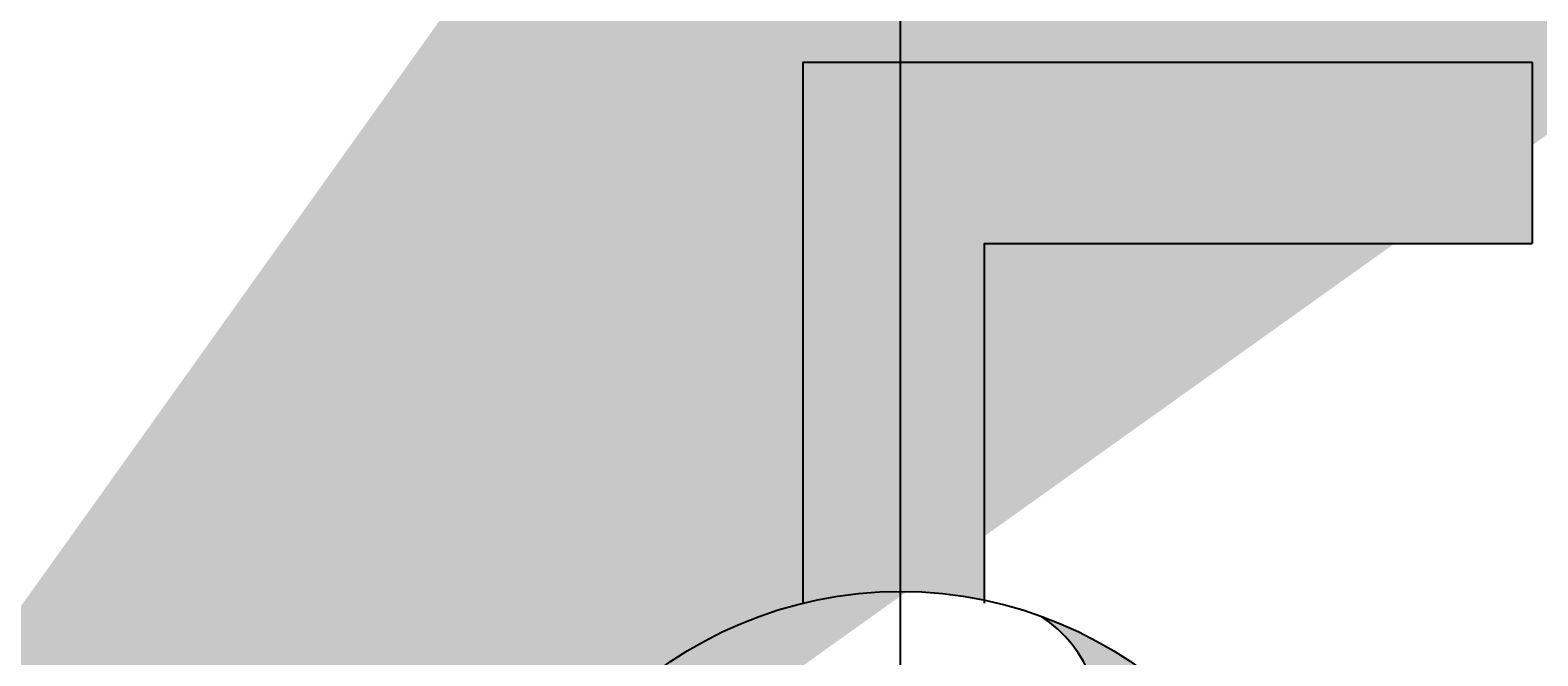
# Model space of a CAD drawing. Units: millimetres. Extents: x -22994 to 29398, y -19990 to 20176.
# Tile 118 of 135: x 204 to 245, y 156 to 174. Entities that reach past the tile are written whole.
import ezdxf

# ---------------------------------------------------------------- set-up
doc = ezdxf.new("R2010")
doc.units = ezdxf.units.MM
doc.header["$MEASUREMENT"] = 0
for name, color, linetype, lineweight in [('M-DIMS', 2, 'Continuous', 18), ('M-EQPM', 7, 'Continuous', 25), ('M-EQPM-PATT', 7, 'Continuous', 18)]:
    doc.layers.add(name, color=color, linetype=linetype, lineweight=lineweight)
doc.styles.get("Standard").update_dxf_attribs({"font": 'arial.ttf'})
doc.dimstyles.get("Standard").update_dxf_attribs({"dimtxt": 0.18, "dimasz": 10000, "dimexe": 0.18, "dimexo": 0.0625, "dimgap": 0.09, "dimtad": 0, "dimtih": 1, "dimtoh": 1, "dimdec": 0, "dimzin": 0, "dimdsep": 46, "dimtxsty": 'Standard', "dimcen": 0.09, "dimadec": 0, "dimazin": 0, "dimtfac": 1, "dimtdec": 0, "dimtofl": 0, "dimtmove": 0, "dimatfit": 3, "dimfxl": 1, "dimtolj": 1, "dimtzin": 0, "dimlwd": 30, "dimarcsym": 0})

# ---------------------------------------------------------------- blocks, each defined once
blk = doc.blocks.new('*D2')
at = {"layer": 'Defpoints', "color": 0, "transparency": 16777216}
for p in [(6.677, 10.271), (290.852, 10.271), (290.852, -5.079)]:
    blk.add_point(p, dxfattribs=at)
at = {"layer": 'M-DIMS', "color": 0, "lineweight": -2, "transparency": 16777216}
for p, q in [((6.677, 10.209), (6.677, -5.259)), ((290.852, 10.209), (290.852, -5.259))]:
    blk.add_line(p, q, dxfattribs=at)
at = {"layer": 'M-DIMS', "color": 0, "lineweight": 30, "transparency": 16777216}
for p, q in [((-9993.323, -5.079), (-19993.323, -5.079)), ((10290.852, -5.079), (20290.852, -5.079))]:
    blk.add_line(p, q, dxfattribs=at)
at = {"layer": 'M-DIMS', "color": 0, "transparency": 16777216}
for points in [[(-9993.323, 1661.588), (-9993.323, -1671.745), (6.677, -5.079)], [(10290.852, 1661.588), (10290.852, -1671.745), (290.852, -5.079)]]:
    blk.add_solid(points, dxfattribs=at)
at = {"layer": 'M-DIMS', "color": 0, "transparency": 16777216, "insert": (148.765, -5.079), "char_height": 0.18, "attachment_point": 5}
blk.add_mtext('\\A1;284.2', dxfattribs=at)
blk = doc.blocks.new('*D3')
at = {"layer": 'Defpoints', "color": 0, "transparency": 16777216}
for p in [(110.265, 204.165), (110.265, 176.366), (95.833, 127.967)]:
    blk.add_point(p, dxfattribs=at)
at = {"layer": 'M-DIMS', "color": 0, "lineweight": 30, "transparency": 16777216}
for p, q in [((-9904.167, 204.165), (-19904.167, 204.165)), ((10110.265, 204.165), (20110.265, 204.165))]:
    blk.add_line(p, q, dxfattribs=at)
at = {"layer": 'M-DIMS', "color": 0, "lineweight": -2, "transparency": 16777216}
for p, q in [((95.833, 128.03), (95.833, 204.345)), ((110.265, 176.429), (110.265, 204.345))]:
    blk.add_line(p, q, dxfattribs=at)
at = {"layer": 'M-DIMS', "color": 0, "transparency": 16777216}
for points in [[(-9904.167, 1870.832), (-9904.167, -1462.501), (95.833, 204.165)], [(10110.265, 1870.832), (10110.265, -1462.501), (110.265, 204.165)]]:
    blk.add_solid(points, dxfattribs=at)
at = {"layer": 'M-DIMS', "color": 0, "transparency": 16777216, "insert": (103.049, 204.165), "char_height": 0.18, "attachment_point": 5}
blk.add_mtext('\\A1;14.432', dxfattribs=at)
blk = doc.blocks.new('*D4')
at = {"layer": 'Defpoints', "color": 0, "transparency": 16777216}
for p in [(116.265, 204.165), (110.265, 176.366), (116.265, 176.366)]:
    blk.add_point(p, dxfattribs=at)
at = {"layer": 'M-DIMS', "color": 0, "lineweight": 30, "transparency": 16777216}
for p, q in [((-9889.735, 204.165), (-19889.735, 204.165)), ((10116.265, 204.165), (20116.265, 204.165))]:
    blk.add_line(p, q, dxfattribs=at)
at = {"layer": 'M-DIMS', "color": 0, "lineweight": -2, "transparency": 16777216}
for p, q in [((110.265, 176.429), (110.265, 204.345)), ((116.265, 176.429), (116.265, 204.345))]:
    blk.add_line(p, q, dxfattribs=at)
at = {"layer": 'M-DIMS', "color": 0, "transparency": 16777216}
for points in [[(-9889.735, 1870.832), (-9889.735, -1462.501), (110.265, 204.165)], [(10116.265, 1870.832), (10116.265, -1462.501), (116.265, 204.165)]]:
    blk.add_solid(points, dxfattribs=at)
at = {"layer": 'M-DIMS', "color": 0, "transparency": 16777216, "insert": (113.265, 204.165), "char_height": 0.18, "attachment_point": 5}
blk.add_mtext('\\A1;6', dxfattribs=at)
blk = doc.blocks.new('*D5')
at = {"layer": 'Defpoints', "color": 0, "transparency": 16777216}
for p in [(181.265, 204.165), (116.265, 176.366), (181.265, 176.366)]:
    blk.add_point(p, dxfattribs=at)
at = {"layer": 'M-DIMS', "color": 0, "lineweight": 30, "transparency": 16777216}
for p, q in [((-9883.735, 204.165), (-19883.735, 204.165)), ((10181.265, 204.165), (20181.265, 204.165))]:
    blk.add_line(p, q, dxfattribs=at)
at = {"layer": 'M-DIMS', "color": 0, "lineweight": -2, "transparency": 16777216}
for p, q in [((116.265, 176.429), (116.265, 204.345)), ((181.265, 176.429), (181.265, 204.345))]:
    blk.add_line(p, q, dxfattribs=at)
at = {"layer": 'M-DIMS', "color": 0, "transparency": 16777216}
for points in [[(-9883.735, 1870.832), (-9883.735, -1462.501), (116.265, 204.165)], [(10181.265, 1870.832), (10181.265, -1462.501), (181.265, 204.165)]]:
    blk.add_solid(points, dxfattribs=at)
at = {"layer": 'M-DIMS', "color": 0, "transparency": 16777216, "insert": (148.765, 204.165), "char_height": 0.18, "attachment_point": 5}
blk.add_mtext('\\A1;65', dxfattribs=at)
blk = doc.blocks.new('*D6')
at = {"layer": 'Defpoints', "color": 0, "transparency": 16777216}
for p in [(187.265, 204.165), (181.265, 176.366), (187.265, 176.366)]:
    blk.add_point(p, dxfattribs=at)
at = {"layer": 'M-DIMS', "color": 0, "lineweight": 30, "transparency": 16777216}
for p, q in [((-9818.735, 204.165), (-19818.735, 204.165)), ((10187.265, 204.165), (20187.265, 204.165))]:
    blk.add_line(p, q, dxfattribs=at)
at = {"layer": 'M-DIMS', "color": 0, "lineweight": -2, "transparency": 16777216}
for p, q in [((181.265, 176.429), (181.265, 204.345)), ((187.265, 176.429), (187.265, 204.345))]:
    blk.add_line(p, q, dxfattribs=at)
at = {"layer": 'M-DIMS', "color": 0, "transparency": 16777216}
for points in [[(-9818.735, 1870.832), (-9818.735, -1462.501), (181.265, 204.165)], [(10187.265, 1870.832), (10187.265, -1462.501), (187.265, 204.165)]]:
    blk.add_solid(points, dxfattribs=at)
at = {"layer": 'M-DIMS', "color": 0, "transparency": 16777216, "insert": (184.265, 204.165), "char_height": 0.18, "attachment_point": 5}
blk.add_mtext('\\A1;6', dxfattribs=at)
blk = doc.blocks.new('*D7')
at = {"layer": 'Defpoints', "color": 0, "transparency": 16777216}
for p in [(201.697, 204.165), (187.265, 176.366), (201.697, 127.967)]:
    blk.add_point(p, dxfattribs=at)
at = {"layer": 'M-DIMS', "color": 0, "lineweight": 30, "transparency": 16777216}
for p, q in [((-9812.735, 204.165), (-19812.735, 204.165)), ((10201.697, 204.165), (20201.697, 204.165))]:
    blk.add_line(p, q, dxfattribs=at)
at = {"layer": 'M-DIMS', "color": 0, "lineweight": -2, "transparency": 16777216}
for p, q in [((187.265, 176.429), (187.265, 204.345)), ((201.697, 128.03), (201.697, 204.345))]:
    blk.add_line(p, q, dxfattribs=at)
at = {"layer": 'M-DIMS', "color": 0, "transparency": 16777216}
for points in [[(-9812.735, 1870.832), (-9812.735, -1462.501), (187.265, 204.165)], [(10201.697, 1870.832), (10201.697, -1462.501), (201.697, 204.165)]]:
    blk.add_solid(points, dxfattribs=at)
at = {"layer": 'M-DIMS', "color": 0, "transparency": 16777216, "insert": (194.481, 204.165), "char_height": 0.18, "attachment_point": 5}
blk.add_mtext('\\A1;14.432', dxfattribs=at)
blk = doc.blocks.new('*D8')
at = {"layer": 'Defpoints', "color": 0, "transparency": 16777216}
for p in [(227.648, 204.165), (227.648, 146.73), (201.697, 127.967)]:
    blk.add_point(p, dxfattribs=at)
at = {"layer": 'M-DIMS', "color": 0, "lineweight": 30, "transparency": 16777216}
for p, q in [((-9798.303, 204.165), (-19798.303, 204.165)), ((10227.648, 204.165), (20227.648, 204.165))]:
    blk.add_line(p, q, dxfattribs=at)
at = {"layer": 'M-DIMS', "color": 0, "lineweight": -2, "transparency": 16777216}
for p, q in [((201.697, 128.03), (201.697, 204.345)), ((227.648, 146.792), (227.648, 204.345))]:
    blk.add_line(p, q, dxfattribs=at)
at = {"layer": 'M-DIMS', "color": 0, "transparency": 16777216}
for points in [[(-9798.303, 1870.832), (-9798.303, -1462.501), (201.697, 204.165)], [(10227.648, 1870.832), (10227.648, -1462.501), (227.648, 204.165)]]:
    blk.add_solid(points, dxfattribs=at)
at = {"layer": 'M-DIMS', "color": 0, "transparency": 16777216, "insert": (214.673, 204.165), "char_height": 0.18, "attachment_point": 5}
blk.add_mtext('\\A1;25.95', dxfattribs=at)
blk = doc.blocks.new('*D9')
at = {"layer": 'Defpoints', "color": 0, "transparency": 16777216}
for p in [(187.265, 176.366), (306.202, 176.366), (290.852, 10.271)]:
    blk.add_point(p, dxfattribs=at)
at = {"layer": 'M-DIMS', "color": 0, "lineweight": 30, "transparency": 16777216}
for p, q in [((306.202, 10176.366), (306.202, 20176.366)), ((306.202, -9989.729), (306.202, -19989.729))]:
    blk.add_line(p, q, dxfattribs=at)
at = {"layer": 'M-DIMS', "color": 0, "lineweight": -2, "transparency": 16777216}
for p, q in [((187.327, 176.366), (306.382, 176.366)), ((290.915, 10.271), (306.382, 10.271))]:
    blk.add_line(p, q, dxfattribs=at)
at = {"layer": 'M-DIMS', "color": 0, "transparency": 16777216}
for points in [[(-1360.465, 10176.366), (1972.869, 10176.366), (306.202, 176.366)], [(-1360.465, -9989.729), (1972.869, -9989.729), (306.202, 10.271)]]:
    blk.add_solid(points, dxfattribs=at)
at = {"layer": 'M-DIMS', "color": 0, "transparency": 16777216, "insert": (306.202, 93.319), "char_height": 0.18, "attachment_point": 5}
blk.add_mtext('\\A1;166.1', dxfattribs=at)
blk = doc.blocks.new('*D10')
at = {"layer": 'Defpoints', "color": 0, "transparency": 16777216}
for p in [(125.65, 136.071), (133.346, 136.071), (133.346, -5.079)]:
    blk.add_point(p, dxfattribs=at)
at = {"layer": 'M-DIMS', "color": 0, "lineweight": -2, "transparency": 16777216}
for p, q in [((125.65, 136.009), (125.65, -5.259)), ((133.346, 136.009), (133.346, -5.259))]:
    blk.add_line(p, q, dxfattribs=at)
at = {"layer": 'M-DIMS', "color": 0, "lineweight": 30, "transparency": 16777216}
for p, q in [((-9874.35, -5.079), (-19874.35, -5.079)), ((10133.346, -5.079), (20133.346, -5.079))]:
    blk.add_line(p, q, dxfattribs=at)
at = {"layer": 'M-DIMS', "color": 0, "transparency": 16777216}
for points in [[(-9874.35, 1661.588), (-9874.35, -1671.745), (125.65, -5.079)], [(10133.346, 1661.588), (10133.346, -1671.745), (133.346, -5.079)]]:
    blk.add_solid(points, dxfattribs=at)
at = {"layer": 'M-DIMS', "color": 0, "transparency": 16777216, "insert": (129.498, -5.079), "char_height": 0.18, "attachment_point": 5}
blk.add_mtext('\\A1;7.696', dxfattribs=at)
blk = doc.blocks.new('*D11')
at = {"layer": 'Defpoints', "color": 0, "transparency": 16777216}
for p in [(133.346, 136.071), (135.65, 136.071), (135.65, -5.079)]:
    blk.add_point(p, dxfattribs=at)
at = {"layer": 'M-DIMS', "color": 0, "lineweight": -2, "transparency": 16777216}
for p, q in [((133.346, 136.009), (133.346, -5.259)), ((135.65, 136.009), (135.65, -5.259))]:
    blk.add_line(p, q, dxfattribs=at)
at = {"layer": 'M-DIMS', "color": 0, "lineweight": 30, "transparency": 16777216}
for p, q in [((-9866.654, -5.079), (-19866.654, -5.079)), ((10135.65, -5.079), (20135.65, -5.079))]:
    blk.add_line(p, q, dxfattribs=at)
at = {"layer": 'M-DIMS', "color": 0, "transparency": 16777216}
for points in [[(-9866.654, 1661.588), (-9866.654, -1671.745), (133.346, -5.079)], [(10135.65, 1661.588), (10135.65, -1671.745), (135.65, -5.079)]]:
    blk.add_solid(points, dxfattribs=at)
at = {"layer": 'M-DIMS', "color": 0, "transparency": 16777216, "insert": (134.498, -5.079), "char_height": 0.18, "attachment_point": 5}
blk.add_mtext('\\A1;2.304', dxfattribs=at)
blk = doc.blocks.new('*D12')
at = {"layer": 'Defpoints', "color": 0, "transparency": 16777216}
for p in [(135.65, 136.071), (145.65, 136.071), (145.65, -5.079)]:
    blk.add_point(p, dxfattribs=at)
at = {"layer": 'M-DIMS', "color": 0, "lineweight": -2, "transparency": 16777216}
for p, q in [((135.65, 136.009), (135.65, -5.259)), ((145.65, 136.009), (145.65, -5.259))]:
    blk.add_line(p, q, dxfattribs=at)
at = {"layer": 'M-DIMS', "color": 0, "lineweight": 30, "transparency": 16777216}
for p, q in [((-9864.35, -5.079), (-19864.35, -5.079)), ((10145.65, -5.079), (20145.65, -5.079))]:
    blk.add_line(p, q, dxfattribs=at)
at = {"layer": 'M-DIMS', "color": 0, "transparency": 16777216}
for points in [[(-9864.35, 1661.588), (-9864.35, -1671.745), (135.65, -5.079)], [(10145.65, 1661.588), (10145.65, -1671.745), (145.65, -5.079)]]:
    blk.add_solid(points, dxfattribs=at)
at = {"layer": 'M-DIMS', "color": 0, "transparency": 16777216, "insert": (140.65, -5.079), "char_height": 0.18, "attachment_point": 5}
blk.add_mtext('\\A1;10', dxfattribs=at)
blk = doc.blocks.new('*D13')
at = {"layer": 'Defpoints', "color": 0, "transparency": 16777216}
for p in [(145.65, 136.071), (155.65, 136.071), (155.65, -5.079)]:
    blk.add_point(p, dxfattribs=at)
at = {"layer": 'M-DIMS', "color": 0, "lineweight": -2, "transparency": 16777216}
for p, q in [((145.65, 136.009), (145.65, -5.259)), ((155.65, 136.009), (155.65, -5.259))]:
    blk.add_line(p, q, dxfattribs=at)
at = {"layer": 'M-DIMS', "color": 0, "lineweight": 30, "transparency": 16777216}
for p, q in [((-9854.35, -5.079), (-19854.35, -5.079)), ((10155.65, -5.079), (20155.65, -5.079))]:
    blk.add_line(p, q, dxfattribs=at)
at = {"layer": 'M-DIMS', "color": 0, "transparency": 16777216}
for points in [[(-9854.35, 1661.588), (-9854.35, -1671.745), (145.65, -5.079)], [(10155.65, 1661.588), (10155.65, -1671.745), (155.65, -5.079)]]:
    blk.add_solid(points, dxfattribs=at)
at = {"layer": 'M-DIMS', "color": 0, "transparency": 16777216, "insert": (150.65, -5.079), "char_height": 0.18, "attachment_point": 5}
blk.add_mtext('\\A1;10', dxfattribs=at)
blk = doc.blocks.new('*D14')
at = {"layer": 'Defpoints', "color": 0, "transparency": 16777216}
for p in [(155.65, 136.071), (165.65, 136.071), (165.65, -5.079)]:
    blk.add_point(p, dxfattribs=at)
at = {"layer": 'M-DIMS', "color": 0, "lineweight": -2, "transparency": 16777216}
for p, q in [((155.65, 136.009), (155.65, -5.259)), ((165.65, 136.009), (165.65, -5.259))]:
    blk.add_line(p, q, dxfattribs=at)
at = {"layer": 'M-DIMS', "color": 0, "lineweight": 30, "transparency": 16777216}
for p, q in [((-9844.35, -5.079), (-19844.35, -5.079)), ((10165.65, -5.079), (20165.65, -5.079))]:
    blk.add_line(p, q, dxfattribs=at)
at = {"layer": 'M-DIMS', "color": 0, "transparency": 16777216}
for points in [[(-9844.35, 1661.588), (-9844.35, -1671.745), (155.65, -5.079)], [(10165.65, 1661.588), (10165.65, -1671.745), (165.65, -5.079)]]:
    blk.add_solid(points, dxfattribs=at)
at = {"layer": 'M-DIMS', "color": 0, "transparency": 16777216, "insert": (160.65, -5.079), "char_height": 0.18, "attachment_point": 5}
blk.add_mtext('\\A1;10', dxfattribs=at)
blk = doc.blocks.new('*D15')
at = {"layer": 'Defpoints', "color": 0, "transparency": 16777216}
for p in [(173.346, 154.788), (173.346, 136.071), (306.202, 136.071)]:
    blk.add_point(p, dxfattribs=at)
at = {"layer": 'M-DIMS', "color": 0, "lineweight": 30, "transparency": 16777216}
for p, q in [((306.202, 10154.788), (306.202, 20154.788)), ((306.202, -9863.929), (306.202, -19863.929))]:
    blk.add_line(p, q, dxfattribs=at)
at = {"layer": 'M-DIMS', "color": 0, "lineweight": -2, "transparency": 16777216}
for p, q in [((173.408, 154.788), (306.382, 154.788)), ((173.408, 136.071), (306.382, 136.071))]:
    blk.add_line(p, q, dxfattribs=at)
at = {"layer": 'M-DIMS', "color": 0, "transparency": 16777216}
for points in [[(-1360.465, 10154.788), (1972.869, 10154.788), (306.202, 154.788)], [(-1360.465, -9863.929), (1972.869, -9863.929), (306.202, 136.071)]]:
    blk.add_solid(points, dxfattribs=at)
at = {"layer": 'M-DIMS', "color": 0, "transparency": 16777216, "insert": (306.202, 145.43), "char_height": 0.18, "attachment_point": 5}
blk.add_mtext('\\A1;18.717', dxfattribs=at)
blk = doc.blocks.new('*D16')
at = {"layer": 'Defpoints', "color": 0, "transparency": 16777216}
for p in [(120.17, 204.165), (110.466, 48.035), (120.17, 48.035)]:
    blk.add_point(p, dxfattribs=at)
at = {"layer": 'M-DIMS', "color": 0, "lineweight": 30, "transparency": 16777216}
for p, q in [((-9889.534, 204.165), (-19889.534, 204.165)), ((10120.17, 204.165), (20120.17, 204.165))]:
    blk.add_line(p, q, dxfattribs=at)
at = {"layer": 'M-DIMS', "color": 0, "lineweight": -2, "transparency": 16777216}
for p, q in [((110.466, 48.097), (110.466, 204.345)), ((120.17, 48.097), (120.17, 204.345))]:
    blk.add_line(p, q, dxfattribs=at)
at = {"layer": 'M-DIMS', "color": 0, "transparency": 16777216}
for points in [[(-9889.534, 1870.832), (-9889.534, -1462.501), (110.466, 204.165)], [(10120.17, 1870.832), (10120.17, -1462.501), (120.17, 204.165)]]:
    blk.add_solid(points, dxfattribs=at)
at = {"layer": 'M-DIMS', "color": 0, "transparency": 16777216, "insert": (115.318, 204.165), "char_height": 0.18, "attachment_point": 5}
blk.add_mtext('\\A1;9.704', dxfattribs=at)
blk = doc.blocks.new('*D17')
at = {"layer": 'Defpoints', "color": 0, "transparency": 16777216}
for p in [(126.17, 204.165), (120.17, 48.035), (126.17, 48.035)]:
    blk.add_point(p, dxfattribs=at)
at = {"layer": 'M-DIMS', "color": 0, "lineweight": 30, "transparency": 16777216}
for p, q in [((-9879.83, 204.165), (-19879.83, 204.165)), ((10126.17, 204.165), (20126.17, 204.165))]:
    blk.add_line(p, q, dxfattribs=at)
at = {"layer": 'M-DIMS', "color": 0, "lineweight": -2, "transparency": 16777216}
for p, q in [((120.17, 48.097), (120.17, 204.345)), ((126.17, 48.097), (126.17, 204.345))]:
    blk.add_line(p, q, dxfattribs=at)
at = {"layer": 'M-DIMS', "color": 0, "transparency": 16777216}
for points in [[(-9879.83, 1870.832), (-9879.83, -1462.501), (120.17, 204.165)], [(10126.17, 1870.832), (10126.17, -1462.501), (126.17, 204.165)]]:
    blk.add_solid(points, dxfattribs=at)
at = {"layer": 'M-DIMS', "color": 0, "transparency": 16777216, "insert": (123.17, 204.165), "char_height": 0.18, "attachment_point": 5}
blk.add_mtext('\\A1;6', dxfattribs=at)
blk = doc.blocks.new('*D18')
at = {"layer": 'Defpoints', "color": 0, "transparency": 16777216}
for p in [(132.17, 204.165), (126.17, 48.035), (132.17, 48.035)]:
    blk.add_point(p, dxfattribs=at)
at = {"layer": 'M-DIMS', "color": 0, "lineweight": 30, "transparency": 16777216}
for p, q in [((-9873.83, 204.165), (-19873.83, 204.165)), ((10132.17, 204.165), (20132.17, 204.165))]:
    blk.add_line(p, q, dxfattribs=at)
at = {"layer": 'M-DIMS', "color": 0, "lineweight": -2, "transparency": 16777216}
for p, q in [((126.17, 48.097), (126.17, 204.345)), ((132.17, 48.097), (132.17, 204.345))]:
    blk.add_line(p, q, dxfattribs=at)
at = {"layer": 'M-DIMS', "color": 0, "transparency": 16777216}
for points in [[(-9873.83, 1870.832), (-9873.83, -1462.501), (126.17, 204.165)], [(10132.17, 1870.832), (10132.17, -1462.501), (132.17, 204.165)]]:
    blk.add_solid(points, dxfattribs=at)
at = {"layer": 'M-DIMS', "color": 0, "transparency": 16777216, "insert": (129.17, 204.165), "char_height": 0.18, "attachment_point": 5}
blk.add_mtext('\\A1;6', dxfattribs=at)
blk = doc.blocks.new('*D19')
at = {"layer": 'Defpoints', "color": 0, "transparency": 16777216}
for p in [(138.17, 204.165), (132.17, 48.035), (138.17, 48.035)]:
    blk.add_point(p, dxfattribs=at)
at = {"layer": 'M-DIMS', "color": 0, "lineweight": 30, "transparency": 16777216}
for p, q in [((-9867.83, 204.165), (-19867.83, 204.165)), ((10138.17, 204.165), (20138.17, 204.165))]:
    blk.add_line(p, q, dxfattribs=at)
at = {"layer": 'M-DIMS', "color": 0, "lineweight": -2, "transparency": 16777216}
for p, q in [((132.17, 48.097), (132.17, 204.345)), ((138.17, 48.097), (138.17, 204.345))]:
    blk.add_line(p, q, dxfattribs=at)
at = {"layer": 'M-DIMS', "color": 0, "transparency": 16777216}
for points in [[(-9867.83, 1870.832), (-9867.83, -1462.501), (132.17, 204.165)], [(10138.17, 1870.832), (10138.17, -1462.501), (138.17, 204.165)]]:
    blk.add_solid(points, dxfattribs=at)
at = {"layer": 'M-DIMS', "color": 0, "transparency": 16777216, "insert": (135.17, 204.165), "char_height": 0.18, "attachment_point": 5}
blk.add_mtext('\\A1;6', dxfattribs=at)
blk = doc.blocks.new('*D20')
at = {"layer": 'Defpoints', "color": 0, "transparency": 16777216}
for p in [(144.17, 204.165), (138.17, 48.035), (144.17, 48.035)]:
    blk.add_point(p, dxfattribs=at)
at = {"layer": 'M-DIMS', "color": 0, "lineweight": 30, "transparency": 16777216}
for p, q in [((-9861.83, 204.165), (-19861.83, 204.165)), ((10144.17, 204.165), (20144.17, 204.165))]:
    blk.add_line(p, q, dxfattribs=at)
at = {"layer": 'M-DIMS', "color": 0, "lineweight": -2, "transparency": 16777216}
for p, q in [((138.17, 48.097), (138.17, 204.345)), ((144.17, 48.097), (144.17, 204.345))]:
    blk.add_line(p, q, dxfattribs=at)
at = {"layer": 'M-DIMS', "color": 0, "transparency": 16777216}
for points in [[(-9861.83, 1870.832), (-9861.83, -1462.501), (138.17, 204.165)], [(10144.17, 1870.832), (10144.17, -1462.501), (144.17, 204.165)]]:
    blk.add_solid(points, dxfattribs=at)
at = {"layer": 'M-DIMS', "color": 0, "transparency": 16777216, "insert": (141.17, 204.165), "char_height": 0.18, "attachment_point": 5}
blk.add_mtext('\\A1;6', dxfattribs=at)
blk = doc.blocks.new('*D21')
at = {"layer": 'Defpoints', "color": 0, "transparency": 16777216}
for p in [(149.116, 204.165), (144.17, 48.035), (149.116, 48.035)]:
    blk.add_point(p, dxfattribs=at)
at = {"layer": 'M-DIMS', "color": 0, "lineweight": 30, "transparency": 16777216}
for p, q in [((-9855.83, 204.165), (-19855.83, 204.165)), ((10149.116, 204.165), (20149.116, 204.165))]:
    blk.add_line(p, q, dxfattribs=at)
at = {"layer": 'M-DIMS', "color": 0, "lineweight": -2, "transparency": 16777216}
for p, q in [((144.17, 48.097), (144.17, 204.345)), ((149.116, 48.097), (149.116, 204.345))]:
    blk.add_line(p, q, dxfattribs=at)
at = {"layer": 'M-DIMS', "color": 0, "transparency": 16777216}
for points in [[(-9855.83, 1870.832), (-9855.83, -1462.501), (144.17, 204.165)], [(10149.116, 1870.832), (10149.116, -1462.501), (149.116, 204.165)]]:
    blk.add_solid(points, dxfattribs=at)
at = {"layer": 'M-DIMS', "color": 0, "transparency": 16777216, "insert": (146.643, 204.165), "char_height": 0.18, "attachment_point": 5}
blk.add_mtext('\\A1;4.945', dxfattribs=at)
blk = doc.blocks.new('*D22')
at = {"layer": 'Defpoints', "color": 0, "transparency": 16777216}
for p in [(149.116, 30.99), (155.116, 30.99), (155.116, -5.079)]:
    blk.add_point(p, dxfattribs=at)
at = {"layer": 'M-DIMS', "color": 0, "lineweight": -2, "transparency": 16777216}
for p, q in [((149.116, 30.927), (149.116, -5.259)), ((155.116, 30.927), (155.116, -5.259))]:
    blk.add_line(p, q, dxfattribs=at)
at = {"layer": 'M-DIMS', "color": 0, "lineweight": 30, "transparency": 16777216}
for p, q in [((-9850.884, -5.079), (-19850.884, -5.079)), ((10155.116, -5.079), (20155.116, -5.079))]:
    blk.add_line(p, q, dxfattribs=at)
at = {"layer": 'M-DIMS', "color": 0, "transparency": 16777216}
for points in [[(-9850.884, 1661.588), (-9850.884, -1671.745), (149.116, -5.079)], [(10155.116, 1661.588), (10155.116, -1671.745), (155.116, -5.079)]]:
    blk.add_solid(points, dxfattribs=at)
at = {"layer": 'M-DIMS', "color": 0, "transparency": 16777216, "insert": (152.116, -5.079), "char_height": 0.18, "attachment_point": 5}
blk.add_mtext('\\A1;6', dxfattribs=at)
blk = doc.blocks.new('*D23')
at = {"layer": 'Defpoints', "color": 0, "transparency": 16777216}
for p in [(155.116, 30.99), (161.116, 30.99), (161.116, -5.079)]:
    blk.add_point(p, dxfattribs=at)
at = {"layer": 'M-DIMS', "color": 0, "lineweight": -2, "transparency": 16777216}
for p, q in [((155.116, 30.927), (155.116, -5.259)), ((161.116, 30.927), (161.116, -5.259))]:
    blk.add_line(p, q, dxfattribs=at)
at = {"layer": 'M-DIMS', "color": 0, "lineweight": 30, "transparency": 16777216}
for p, q in [((-9844.884, -5.079), (-19844.884, -5.079)), ((10161.116, -5.079), (20161.116, -5.079))]:
    blk.add_line(p, q, dxfattribs=at)
at = {"layer": 'M-DIMS', "color": 0, "transparency": 16777216}
for points in [[(-9844.884, 1661.588), (-9844.884, -1671.745), (155.116, -5.079)], [(10161.116, 1661.588), (10161.116, -1671.745), (161.116, -5.079)]]:
    blk.add_solid(points, dxfattribs=at)
at = {"layer": 'M-DIMS', "color": 0, "transparency": 16777216, "insert": (158.116, -5.079), "char_height": 0.18, "attachment_point": 5}
blk.add_mtext('\\A1;6', dxfattribs=at)
blk = doc.blocks.new('*D24')
at = {"layer": 'Defpoints', "color": 0, "transparency": 16777216}
for p in [(161.116, 30.99), (166.439, 30.99), (166.439, -5.079)]:
    blk.add_point(p, dxfattribs=at)
at = {"layer": 'M-DIMS', "color": 0, "lineweight": -2, "transparency": 16777216}
for p, q in [((161.116, 30.927), (161.116, -5.259)), ((166.439, 30.927), (166.439, -5.259))]:
    blk.add_line(p, q, dxfattribs=at)
at = {"layer": 'M-DIMS', "color": 0, "lineweight": 30, "transparency": 16777216}
for p, q in [((-9838.884, -5.079), (-19838.884, -5.079)), ((10166.439, -5.079), (20166.439, -5.079))]:
    blk.add_line(p, q, dxfattribs=at)
at = {"layer": 'M-DIMS', "color": 0, "transparency": 16777216}
for points in [[(-9838.884, 1661.588), (-9838.884, -1671.745), (161.116, -5.079)], [(10166.439, 1661.588), (10166.439, -1671.745), (166.439, -5.079)]]:
    blk.add_solid(points, dxfattribs=at)
at = {"layer": 'M-DIMS', "color": 0, "transparency": 16777216, "insert": (163.777, -5.079), "char_height": 0.18, "attachment_point": 5}
blk.add_mtext('\\A1;5.323', dxfattribs=at)
blk = doc.blocks.new('*D25')
at = {"layer": 'Defpoints', "color": 0, "transparency": 16777216}
for p in [(166.439, 30.99), (172.439, 30.99), (172.439, -5.079)]:
    blk.add_point(p, dxfattribs=at)
at = {"layer": 'M-DIMS', "color": 0, "lineweight": -2, "transparency": 16777216}
for p, q in [((166.439, 30.927), (166.439, -5.259)), ((172.439, 30.927), (172.439, -5.259))]:
    blk.add_line(p, q, dxfattribs=at)
at = {"layer": 'M-DIMS', "color": 0, "lineweight": 30, "transparency": 16777216}
for p, q in [((-9833.561, -5.079), (-19833.561, -5.079)), ((10172.439, -5.079), (20172.439, -5.079))]:
    blk.add_line(p, q, dxfattribs=at)
at = {"layer": 'M-DIMS', "color": 0, "transparency": 16777216}
for points in [[(-9833.561, 1661.588), (-9833.561, -1671.745), (166.439, -5.079)], [(10172.439, 1661.588), (10172.439, -1671.745), (172.439, -5.079)]]:
    blk.add_solid(points, dxfattribs=at)
at = {"layer": 'M-DIMS', "color": 0, "transparency": 16777216, "insert": (169.439, -5.079), "char_height": 0.18, "attachment_point": 5}
blk.add_mtext('\\A1;6', dxfattribs=at)
blk = doc.blocks.new('*D26')
at = {"layer": 'Defpoints', "color": 0, "transparency": 16777216}
for p in [(172.439, 30.99), (178.439, 30.99), (178.439, -5.079)]:
    blk.add_point(p, dxfattribs=at)
at = {"layer": 'M-DIMS', "color": 0, "lineweight": -2, "transparency": 16777216}
for p, q in [((172.439, 30.927), (172.439, -5.259)), ((178.439, 30.927), (178.439, -5.259))]:
    blk.add_line(p, q, dxfattribs=at)
at = {"layer": 'M-DIMS', "color": 0, "lineweight": 30, "transparency": 16777216}
for p, q in [((-9827.561, -5.079), (-19827.561, -5.079)), ((10178.439, -5.079), (20178.439, -5.079))]:
    blk.add_line(p, q, dxfattribs=at)
at = {"layer": 'M-DIMS', "color": 0, "transparency": 16777216}
for points in [[(-9827.561, 1661.588), (-9827.561, -1671.745), (172.439, -5.079)], [(10178.439, 1661.588), (10178.439, -1671.745), (178.439, -5.079)]]:
    blk.add_solid(points, dxfattribs=at)
at = {"layer": 'M-DIMS', "color": 0, "transparency": 16777216, "insert": (175.439, -5.079), "char_height": 0.18, "attachment_point": 5}
blk.add_mtext('\\A1;6', dxfattribs=at)
blk = doc.blocks.new('*D27')
at = {"layer": 'Defpoints', "color": 0, "transparency": 16777216}
for p in [(178.439, 30.99), (188.117, 30.99), (188.117, -5.079)]:
    blk.add_point(p, dxfattribs=at)
at = {"layer": 'M-DIMS', "color": 0, "lineweight": -2, "transparency": 16777216}
for p, q in [((178.439, 30.927), (178.439, -5.259)), ((188.117, 30.927), (188.117, -5.259))]:
    blk.add_line(p, q, dxfattribs=at)
at = {"layer": 'M-DIMS', "color": 0, "lineweight": 30, "transparency": 16777216}
for p, q in [((-9821.561, -5.079), (-19821.561, -5.079)), ((10188.117, -5.079), (20188.117, -5.079))]:
    blk.add_line(p, q, dxfattribs=at)
at = {"layer": 'M-DIMS', "color": 0, "transparency": 16777216}
for points in [[(-9821.561, 1661.588), (-9821.561, -1671.745), (178.439, -5.079)], [(10188.117, 1661.588), (10188.117, -1671.745), (188.117, -5.079)]]:
    blk.add_solid(points, dxfattribs=at)
at = {"layer": 'M-DIMS', "color": 0, "transparency": 16777216, "insert": (183.278, -5.079), "char_height": 0.18, "attachment_point": 5}
blk.add_mtext('\\A1;9.679', dxfattribs=at)
blk = doc.blocks.new('*D28')
at = {"layer": 'Defpoints', "color": 0, "transparency": 16777216}
for p in [(188.117, 48.035), (306.202, 48.035), (188.117, 30.99)]:
    blk.add_point(p, dxfattribs=at)
at = {"layer": 'M-DIMS', "color": 0, "lineweight": 30, "transparency": 16777216}
for p, q in [((306.202, 10048.035), (306.202, 20048.035)), ((306.202, -9969.01), (306.202, -19969.01))]:
    blk.add_line(p, q, dxfattribs=at)
at = {"layer": 'M-DIMS', "color": 0, "lineweight": -2, "transparency": 16777216}
for p, q in [((188.18, 48.035), (306.382, 48.035)), ((188.18, 30.99), (306.382, 30.99))]:
    blk.add_line(p, q, dxfattribs=at)
at = {"layer": 'M-DIMS', "color": 0, "transparency": 16777216}
for points in [[(-1360.465, 10048.035), (1972.869, 10048.035), (306.202, 48.035)], [(-1360.465, -9969.01), (1972.869, -9969.01), (306.202, 30.99)]]:
    blk.add_solid(points, dxfattribs=at)
at = {"layer": 'M-DIMS', "color": 0, "transparency": 16777216, "insert": (306.202, 39.512), "char_height": 0.18, "attachment_point": 5}
blk.add_mtext('\\A1;17.045', dxfattribs=at)
blk = doc.blocks.new('*D29')
at = {"layer": 'Defpoints', "color": 0, "transparency": 16777216}
for p in [(36.801, 80.045), (64.03, 80.045)]:
    blk.add_point(p, dxfattribs=at)
at = {"layer": 'M-DIMS', "color": 0, "lineweight": -2, "transparency": 16777216}
for p, q in [((50.325, 80.045), (50.505, 80.045)), ((50.415, 79.955), (50.415, 80.135))]:
    blk.add_line(p, q, dxfattribs=at)
at = {"layer": 'M-DIMS', "color": 0, "lineweight": 30, "transparency": 16777216}
blk.add_line((20064.03, 80.03), (10064.03, 80.038), dxfattribs=at)
at = {"layer": 'M-DIMS', "color": 0, "transparency": 16777216}
blk.add_solid([(10064.031, 1746.704), (10064.028, -1586.629), (64.03, 80.045)], dxfattribs=at)
at = {"layer": 'M-DIMS', "color": 0, "transparency": 16777216, "insert": (20064.521, 80.03), "char_height": 0.18, "attachment_point": 5}
blk.add_mtext('\\A1;∅27.23', dxfattribs=at)
blk = doc.blocks.new('*D30')
at = {"layer": 'Defpoints', "color": 0, "transparency": 16777216}
for p in [(216.315, 146.729), (238.982, 146.73)]:
    blk.add_point(p, dxfattribs=at)
at = {"layer": 'M-DIMS', "color": 0, "lineweight": 30, "transparency": 16777216}
blk.add_line((20238.982, 147.496), (10238.982, 147.113), dxfattribs=at)
at = {"layer": 'M-DIMS', "color": 0, "lineweight": -2, "transparency": 16777216}
for p, q in [((227.558, 146.73), (227.738, 146.73)), ((227.648, 146.64), (227.648, 146.82))]:
    blk.add_line(p, q, dxfattribs=at)
at = {"layer": 'M-DIMS', "color": 0, "transparency": 16777216}
blk.add_solid([(10238.918, 1813.78), (10239.046, -1519.554), (238.982, 146.73)], dxfattribs=at)
at = {"layer": 'M-DIMS', "color": 0, "transparency": 16777216, "insert": (20239.544, 147.496), "char_height": 0.18, "attachment_point": 5}
blk.add_mtext('\\A1;∅22.667', dxfattribs=at)
blk = doc.blocks.new('*D31')
at = {"layer": 'Defpoints', "color": 0, "transparency": 16777216}
for p in [(223.164, 146.729), (232.133, 146.73)]:
    blk.add_point(p, dxfattribs=at)
at = {"layer": 'M-DIMS', "color": 0, "lineweight": 30, "transparency": 16777216}
blk.add_line((20232.133, 148.666), (10232.133, 147.698), dxfattribs=at)
at = {"layer": 'M-DIMS', "color": 0, "lineweight": -2, "transparency": 16777216}
for p, q in [((227.558, 146.73), (227.738, 146.73)), ((227.648, 146.64), (227.648, 146.82))]:
    blk.add_line(p, q, dxfattribs=at)
at = {"layer": 'M-DIMS', "color": 0, "transparency": 16777216}
blk.add_solid([(10231.971, 1814.364), (10232.294, -1518.969), (232.133, 146.73)], dxfattribs=at)
at = {"layer": 'M-DIMS', "color": 0, "transparency": 16777216, "insert": (20232.625, 148.666), "char_height": 0.18, "attachment_point": 5}
blk.add_mtext('\\A1;∅8.969', dxfattribs=at)
blk = doc.blocks.new('*D34')
at = {"layer": 'Defpoints', "color": 0, "transparency": 16777216}
for p in [(178.58, 122.895), (176.812, 121.128)]:
    blk.add_point(p, dxfattribs=at)
at = {"layer": 'M-DIMS', "color": 0, "lineweight": 30, "transparency": 16777216}
for p, q in [((14322.436, 14263.311), (7250.508, 7193.103)), ((24322.436, 14263.311), (14322.436, 14263.311))]:
    blk.add_line(p, q, dxfattribs=at)
at = {"layer": 'M-DIMS', "color": 0, "lineweight": -2, "transparency": 16777216}
for p, q in [((176.722, 121.128), (176.902, 121.128)), ((176.812, 121.038), (176.812, 121.218))]:
    blk.add_line(p, q, dxfattribs=at)
at = {"layer": 'M-DIMS', "color": 0, "transparency": 16777216}
blk.add_solid([(6072.14, 8371.758), (8428.876, 6014.448), (178.58, 122.895)], dxfattribs=at)
at = {"layer": 'M-DIMS', "color": 0, "transparency": 16777216, "insert": (24322.97, 14263.311), "char_height": 0.18, "attachment_point": 5}
blk.add_mtext('\\A1;6X R2.5', dxfattribs=at)
blk = doc.blocks.new('*D36')
at = {"layer": 'Defpoints', "color": 0, "transparency": 16777216}
for p in [(46.39, 31.303), (46.387, 26.593)]:
    blk.add_point(p, dxfattribs=at)
at = {"layer": 'M-DIMS', "color": 0, "lineweight": 30, "transparency": 16777216}
for p, q in [((57.15, 20031.301), (51.77, 10031.302)), ((10057.15, 20031.301), (57.15, 20031.301))]:
    blk.add_line(p, q, dxfattribs=at)
at = {"layer": 'M-DIMS', "color": 0, "lineweight": -2, "transparency": 16777216}
for p, q in [((46.299, 28.948), (46.479, 28.948)), ((46.389, 28.858), (46.389, 29.038))]:
    blk.add_line(p, q, dxfattribs=at)
at = {"layer": 'M-DIMS', "color": 0, "transparency": 16777216}
blk.add_solid([(-1614.896, 10032.199), (1718.436, 10030.405), (46.39, 31.303)], dxfattribs=at)
at = {"layer": 'M-DIMS', "color": 0, "transparency": 16777216, "insert": (10057.554, 20031.301), "char_height": 0.18, "attachment_point": 5}
blk.add_mtext('\\A1;∅4.71', dxfattribs=at)
blk = doc.blocks.new('*D37')
at = {"layer": 'Defpoints', "color": 0, "transparency": 16777216}
for p in [(54.834, 118.615), (59.494, 118.614)]:
    blk.add_point(p, dxfattribs=at)
at = {"layer": 'M-DIMS', "color": 0, "lineweight": -2, "transparency": 16777216}
for p, q in [((57.074, 118.614), (57.254, 118.614)), ((57.164, 118.524), (57.164, 118.704))]:
    blk.add_line(p, q, dxfattribs=at)
at = {"layer": 'M-DIMS', "color": 0, "lineweight": 30, "transparency": 16777216}
blk.add_line((20059.493, 116.253), (10059.494, 117.434), dxfattribs=at)
at = {"layer": 'M-DIMS', "color": 0, "transparency": 16777216}
blk.add_solid([(10059.69, 1784.1), (10059.297, -1549.233), (59.494, 118.614)], dxfattribs=at)
at = {"layer": 'M-DIMS', "color": 0, "transparency": 16777216, "insert": (20059.985, 116.253), "char_height": 0.18, "attachment_point": 5}
blk.add_mtext('\\A1;∅4.659', dxfattribs=at)

msp = doc.modelspace()

# ---------------------------------------------------------------- hatches: boundary and pattern name
at = {"layer": 'M-EQPM-PATT'}
h = msp.add_hatch(color=256, dxfattribs=at)
h.set_gradient(color1=(128, 128, 128), color2=(128, 128, 128), tint=1)
h.paths.add_polyline_path([(88.0003, 148.1301), (88.0003, 143.1301), (104.9278, 143.1301), (107.9269, 148.1301)])
h.paths.add_polyline_path([(189.6025, 148.1301), (192.6016, 143.1301), (216.9016, 143.1301, -0.0809736), (216.3148, 146.7296, -0.0309822), (216.4017, 148.1301)])
h.paths.add_polyline_path([(229.9653, 167.6546), (245.0476, 167.6546), (245.0476, 172.6546), (224.9653, 172.6546), (224.9653, 157.741, -0.1116822), (229.9653, 157.8239)])
h.paths.add_polyline_path([(36.3887, 21.6644), (36.3887, 16.6063), (56.3887, 16.6063), (56.3887, 21.6644)])
h = msp.add_hatch(color=256, dxfattribs=at)
h.set_gradient(color1=(0, 0, 255), color2=(244, 238, 81), tint=1, name='CYLINDER')
h.paths.add_polyline_path([(232.1163, 147.1148, 0.7475711), (238.8087, 148.7044, 0.2679492), (231.5183, 157.3821, -0.7475711), (229.5488, 150.7914, -0.2679492)])
h.paths.add_polyline_path([(216.3148, 146.7296, 0.0438131), (216.4882, 144.7547, -0.7475711), (223.1807, 146.3444, -0.0215046), (223.1641, 146.7296, -0.2450326), (225.081, 150.4062, 0.7475711), (220.3581, 155.4072, 0.2215353)])
h.paths.add_polyline_path([(234.9389, 138.0519, -0.7475711), (230.216, 143.053, -0.2679492), (225.7482, 142.6678, 0.7475711), (223.7786, 136.0771, 0.2679492)])

# ---------------------------------------------------------------- linework, layer by layer
at = {"layer": 'M-EQPM'}
msp.add_line((245.0476, 172.6546), (245.0476, 167.6546), dxfattribs=at)
for points in [[(224.9653, 157.741), (224.9653, 172.6546), (245.0476, 172.6546)], [(229.9653, 157.741), (229.9653, 167.6546), (245.0476, 167.6546)]]:
    msp.add_lwpolyline(points, dxfattribs=at)
msp.add_circle((227.6485, 146.7296), 11.3336, dxfattribs=at)
msp.add_arc((229.5613, 154.3773), 3.5859, 269.80022, 56.92313, dxfattribs=at)

# ---------------------------------------------------------------- dimensions: what is measured, and where the dimension line sits
at = {"layer": 'M-DIMS'}
for base, p1, p2, override, picture, middle in [((306.202, 176.3662), (290.852, 10.2713), (187.2647, 176.3662), {"dimdec": 1, "dimlfac": 1, "dimrnd": 0, "dimzin": 0, "dimdsep": 46, "dimlunit": 2}, '*D9', (306.202, 93.3187)), ((306.202, 136.0713), (173.3459, 154.788), (173.3459, 136.0713), {"dimdec": 3, "dimlfac": 1, "dimrnd": 0, "dimzin": 0, "dimdsep": 46, "dimlunit": 2}, '*D15', (306.202, 145.4297)), ((306.202, 48.0349), (188.1175, 30.9895), (188.1175, 48.0349), {"dimdec": 3, "dimlfac": 1, "dimrnd": 0, "dimzin": 0, "dimdsep": 46, "dimlunit": 2}, '*D28', (306.202, 39.5122))]:
    dim = msp.add_linear_dim(base=base, p1=p1, p2=p2, angle=90, dimstyle='Standard', override=override, dxfattribs=at)
    dim.commit()
    dim.dimension.update_dxf_attribs({"geometry": picture, "text_midpoint": middle})
for p1, p2, override, picture, middle in [((46.3875, 26.5934), (46.39, 31.3035), {"dimdec": 2, "dimlfac": 1, "dimrnd": 0, "dimzin": 0, "dimdsep": 46, "dimlunit": 2}, '*D36', (10057.5542, 20031.3006)), ((223.1641, 146.7291), (232.1328, 146.73), {"dimdec": 3, "dimlfac": 1, "dimrnd": 0, "dimzin": 0, "dimdsep": 46, "dimlunit": 2}, '*D31', (20232.1327, 148.6656)), ((216.3148, 146.7291), (238.9821, 146.73), {"dimdec": 3, "dimlfac": 1, "dimrnd": 0, "dimzin": 0, "dimdsep": 46, "dimlunit": 2}, '*D30', (20238.9821, 147.4959))]:
    dim = msp.add_diameter_dim_2p(p1=p1, p2=p2, dimstyle='Standard', override=override, dxfattribs=at)
    dim.commit()
    dim.dimension.update_dxf_attribs({"geometry": picture, "text_midpoint": middle, "dimtype": 163})
dim = msp.add_radius_dim(center=(176.8123, 121.1277), mpoint=(178.5802, 122.8952), text='6X <>', dimstyle='Standard', override={"dimdec": 1, "dimlfac": 1, "dimrnd": 0, "dimzin": 0, "dimdsep": 46, "dimlunit": 2}, dxfattribs=at)
dim.commit()
dim.dimension.update_dxf_attribs({"geometry": '*D34', "text_midpoint": (24322.9703, 14263.3108)})
for base, p1, p2, override, picture, middle in [((110.2647, 204.1654), (95.8327, 127.967), (110.2647, 176.3662), {"dimdec": 3, "dimlfac": 1, "dimrnd": 0, "dimzin": 0, "dimdsep": 46, "dimlunit": 2}, '*D3', (103.0487, 204.1654)), ((116.2647, 204.1654), (110.2647, 176.3662), (116.2647, 176.3662), {"dimdec": 0, "dimlfac": 1, "dimrnd": 0, "dimzin": 0, "dimdsep": 46, "dimlunit": 2}, '*D4', (113.2647, 204.1654)), ((120.1702, 204.1654), (110.4658, 48.0349), (120.1702, 48.0349), {"dimdec": 3, "dimlfac": 1, "dimrnd": 0, "dimzin": 0, "dimdsep": 46, "dimlunit": 2}, '*D16', (115.318, 204.1654)), ((181.2647, 204.1654), (116.2647, 176.3662), (181.2647, 176.3662), {"dimdec": 0, "dimlfac": 1, "dimrnd": 0, "dimzin": 0, "dimdsep": 46, "dimlunit": 2}, '*D5', (148.7647, 204.1654)), ((126.1702, 204.1654), (120.1702, 48.0349), (126.1702, 48.0349), {"dimdec": 0, "dimlfac": 1, "dimrnd": 0, "dimzin": 0, "dimdsep": 46, "dimlunit": 2}, '*D17', (123.1702, 204.1654)), ((132.1702, 204.1654), (126.1702, 48.0349), (132.1702, 48.0349), {"dimdec": 0, "dimlfac": 1, "dimrnd": 0, "dimzin": 0, "dimdsep": 46, "dimlunit": 2}, '*D18', (129.1702, 204.1654)), ((138.1702, 204.1654), (132.1702, 48.0349), (138.1702, 48.0349), {"dimdec": 0, "dimlfac": 1, "dimrnd": 0, "dimzin": 0, "dimdsep": 46, "dimlunit": 2}, '*D19', (135.1702, 204.1654)), ((144.1702, 204.1654), (138.1702, 48.0349), (144.1702, 48.0349), {"dimdec": 0, "dimlfac": 1, "dimrnd": 0, "dimzin": 0, "dimdsep": 46, "dimlunit": 2}, '*D20', (141.1702, 204.1654)), ((149.11567, 204.16539), (144.17023, 48.03494), (149.11567, 48.03494), {"dimdec": 3, "dimlfac": 1, "dimrnd": 0, "dimzin": 0, "dimdsep": 46, "dimlunit": 2}, '*D21', (146.64295, 204.16539)), ((187.2647, 204.1654), (181.2647, 176.3662), (187.2647, 176.3662), {"dimdec": 0, "dimlfac": 1, "dimrnd": 0, "dimzin": 0, "dimdsep": 46, "dimlunit": 2}, '*D6', (184.2647, 204.1654)), ((201.6967, 204.1654), (187.2647, 176.3662), (201.6967, 127.967), {"dimdec": 3, "dimlfac": 1, "dimrnd": 0, "dimzin": 0, "dimdsep": 46, "dimlunit": 2}, '*D7', (194.4807, 204.1654)), ((227.6485, 204.1654), (201.6967, 127.967), (227.6485, 146.7296), {"dimdec": 2, "dimlfac": 1, "dimrnd": 0, "dimzin": 0, "dimdsep": 46, "dimlunit": 2}, '*D8', (214.6726, 204.1654)), ((290.852, -5.0787), (6.6773, 10.2713), (290.852, 10.2713), {"dimdec": 1, "dimlfac": 1, "dimrnd": 0, "dimzin": 0, "dimdsep": 46, "dimlunit": 2}, '*D2', (148.7647, -5.0787)), ((133.3459, -5.0787), (125.6498, 136.0713), (133.3459, 136.0713), {"dimdec": 3, "dimlfac": 1, "dimrnd": 0, "dimzin": 0, "dimdsep": 46, "dimlunit": 2}, '*D10', (129.4978, -5.0787)), ((135.6498, -5.0787), (133.3459, 136.0713), (135.6498, 136.0713), {"dimdec": 3, "dimlfac": 1, "dimrnd": 0, "dimzin": 0, "dimdsep": 46, "dimlunit": 2}, '*D11', (134.4978, -5.0787)), ((145.6498, -5.0787), (135.6498, 136.0713), (145.6498, 136.0713), {"dimdec": 0, "dimlfac": 1, "dimrnd": 0, "dimzin": 0, "dimdsep": 46, "dimlunit": 2}, '*D12', (140.6498, -5.0787)), ((155.6498, -5.0787), (145.6498, 136.0713), (155.6498, 136.0713), {"dimdec": 0, "dimlfac": 1, "dimrnd": 0, "dimzin": 0, "dimdsep": 46, "dimlunit": 2}, '*D13', (150.6498, -5.0787)), ((155.1157, -5.0787), (149.1157, 30.9895), (155.1157, 30.9895), {"dimdec": 0, "dimlfac": 1, "dimrnd": 0, "dimzin": 0, "dimdsep": 46, "dimlunit": 2}, '*D22', (152.1157, -5.0787)), ((161.1157, -5.0787), (155.1157, 30.9895), (161.1157, 30.9895), {"dimdec": 0, "dimlfac": 1, "dimrnd": 0, "dimzin": 0, "dimdsep": 46, "dimlunit": 2}, '*D23', (158.1157, -5.0787)), ((165.6498, -5.0787), (155.6498, 136.0713), (165.6498, 136.0713), {"dimdec": 0, "dimlfac": 1, "dimrnd": 0, "dimzin": 0, "dimdsep": 46, "dimlunit": 2}, '*D14', (160.6498, -5.0787)), ((166.4387, -5.0787), (161.1157, 30.9895), (166.4387, 30.9895), {"dimdec": 3, "dimlfac": 1, "dimrnd": 0, "dimzin": 0, "dimdsep": 46, "dimlunit": 2}, '*D24', (163.7772, -5.0787)), ((172.4387, -5.0787), (166.4387, 30.9895), (172.4387, 30.9895), {"dimdec": 0, "dimlfac": 1, "dimrnd": 0, "dimzin": 0, "dimdsep": 46, "dimlunit": 2}, '*D25', (169.4387, -5.0787)), ((178.4387, -5.0787), (172.4387, 30.9895), (178.4387, 30.9895), {"dimdec": 0, "dimlfac": 1, "dimrnd": 0, "dimzin": 0, "dimdsep": 46, "dimlunit": 2}, '*D26', (175.4387, -5.0787)), ((188.1175, -5.0787), (178.4387, 30.9895), (188.1175, 30.9895), {"dimdec": 3, "dimlfac": 1, "dimrnd": 0, "dimzin": 0, "dimdsep": 46, "dimlunit": 2}, '*D27', (183.2781, -5.0787))]:
    dim = msp.add_linear_dim(base=base, p1=p1, p2=p2, dimstyle='Standard', override=override, dxfattribs=at)
    dim.commit()
    dim.dimension.update_dxf_attribs({"geometry": picture, "text_midpoint": middle})
for p1, p2, override, picture, middle in [((54.8343, 118.6145), (59.4936, 118.614), {"dimdec": 3, "dimlfac": 1, "dimrnd": 0, "dimzin": 0, "dimdsep": 46, "dimlunit": 2}, '*D37', (20059.4934, 116.2531)), ((36.8006, 80.045), (64.0296, 80.045), {"dimdec": 2, "dimlfac": 1, "dimrnd": 0, "dimzin": 0, "dimdsep": 46, "dimlunit": 2}, '*D29', (20064.0296, 80.0303))]:
    dim = msp.add_diameter_dim_2p(p1=p1, p2=p2, dimstyle='Standard', override=override, dxfattribs=at)
    dim.commit()
    dim.dimension.update_dxf_attribs({"geometry": picture, "text_midpoint": middle})

doc.saveas('drawing.dxf')
